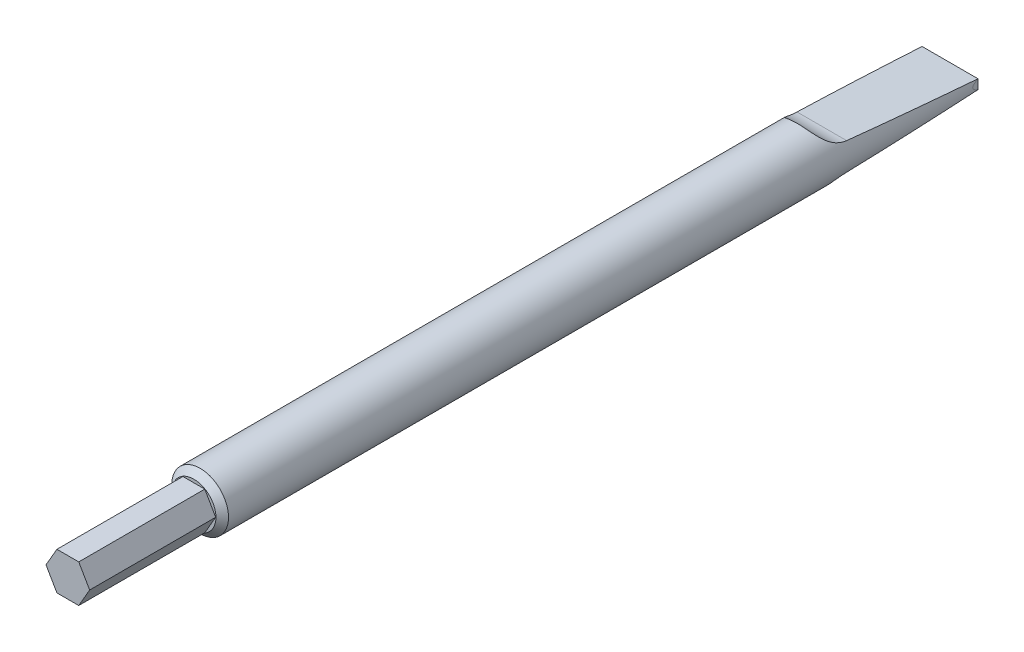
ISO-10303-21;
HEADER;
FILE_DESCRIPTION(('STEP AP214'),'2;1');
FILE_NAME('part.step','',(''),(''),'','','');
FILE_SCHEMA(('AUTOMOTIVE_DESIGN { 1 0 10303 214 1 1 1 1 }'));
ENDSEC;
DATA;
#1=APPLICATION_CONTEXT('core data for automotive mechanical design processes');
#2=APPLICATION_PROTOCOL_DEFINITION('international standard','automotive_design',2000,#1);
#3=PRODUCT_CONTEXT('',#1,'mechanical');
#4=PRODUCT('Part','Part','',(#3));
#5=PRODUCT_RELATED_PRODUCT_CATEGORY('part','',(#4));
#6=PRODUCT_DEFINITION_FORMATION('','',#4);
#7=PRODUCT_DEFINITION_CONTEXT('part definition',#1,'design');
#8=PRODUCT_DEFINITION('design','',#6,#7);
#9=PRODUCT_DEFINITION_SHAPE('','',#8);
#10=(LENGTH_UNIT() NAMED_UNIT(*) SI_UNIT(.MILLI.,.METRE.));
#11=(NAMED_UNIT(*) PLANE_ANGLE_UNIT() SI_UNIT($,.RADIAN.));
#12=(NAMED_UNIT(*) SI_UNIT($,.STERADIAN.) SOLID_ANGLE_UNIT());
#13=UNCERTAINTY_MEASURE_WITH_UNIT(LENGTH_MEASURE(1.E-05),#10,'distance_accuracy_value','');
#14=(GEOMETRIC_REPRESENTATION_CONTEXT(3) GLOBAL_UNCERTAINTY_ASSIGNED_CONTEXT((#13)) GLOBAL_UNIT_ASSIGNED_CONTEXT((#10,
#11,#12)) REPRESENTATION_CONTEXT('',''));
#15=CARTESIAN_POINT('',(0.,0.,0.));
#16=DIRECTION('',(0.,0.,1.));
#17=DIRECTION('',(1.,0.,0.));
#18=AXIS2_PLACEMENT_3D('',#15,#16,#17);
#19=CARTESIAN_POINT('',(0.,0.,-140.));
#20=DIRECTION('',(0.,0.,1.));
#21=DIRECTION('',(1.,0.,0.));
#22=AXIS2_PLACEMENT_3D('',#19,#20,#21);
#23=CYLINDRICAL_SURFACE('',#22,4.5);
#24=CARTESIAN_POINT('',(0.,0.,-21.));
#25=DIRECTION('',(0.,0.,1.));
#26=DIRECTION('',(1.,0.,0.));
#27=AXIS2_PLACEMENT_3D('',#24,#25,#26);
#28=CIRCLE('',#27,4.5);
#29=CARTESIAN_POINT('',(4.5,0.,-21.));
#30=VERTEX_POINT('',#29);
#31=EDGE_CURVE('E199',#30,#30,#28,.F.);
#32=ORIENTED_EDGE('',*,*,#31,.T.);
#33=EDGE_LOOP('',(#32));
#34=FACE_BOUND('',#33,.T.);
#35=CARTESIAN_POINT('',(0.,0.,-150.725499692534));
#36=DIRECTION('',(0.,-0.997564050259824,0.0697564737441254));
#37=DIRECTION('',(0.,0.0697564737441254,0.997564050259824));
#38=AXIS2_PLACEMENT_3D('',#35,#36,#37);
#39=ELLIPSE('',#38,64.5101416179165,4.5);
#40=CARTESIAN_POINT('',(4.43705983732471,0.75,-140.));
#41=VERTEX_POINT('',#40);
#42=CARTESIAN_POINT('',(3.94060843870063,2.17292547797695,-119.651217631279));
#43=VERTEX_POINT('',#42);
#44=EDGE_CURVE('E134',#41,#43,#39,.T.);
#45=ORIENTED_EDGE('',*,*,#44,.T.);
#46=CARTESIAN_POINT('',(3.94060843870063,2.17292547797695,-119.651217631279));
#47=CARTESIAN_POINT('',(3.93613453836127,2.18097697918258,-119.535820622681));
#48=CARTESIAN_POINT('',(3.92947094474121,2.19306262577348,-119.420781980209));
#49=CARTESIAN_POINT('',(3.91143990386196,2.22509503569858,-119.192142075211));
#50=CARTESIAN_POINT('',(3.90007100119166,2.24504423123616,-119.078541268641));
#51=CARTESIAN_POINT('',(3.87225058788964,2.29268834893347,-118.853110956475));
#52=CARTESIAN_POINT('',(3.8557785222487,2.32041455254767,-118.741290572735));
#53=CARTESIAN_POINT('',(3.81728624165493,2.38320927692897,-118.520713395312));
#54=CARTESIAN_POINT('',(3.7952665438402,2.41827711327371,-118.411956317124));
#55=CARTESIAN_POINT('',(3.74503067779343,2.49536896839162,-118.197992726652));
#56=CARTESIAN_POINT('',(3.71679509883591,2.53741467384938,-118.092798554982));
#57=CARTESIAN_POINT('',(3.65353870193094,2.62767774279538,-117.887206844789));
#58=CARTESIAN_POINT('',(3.61851845768965,2.6758945843401,-117.786808901595));
#59=CARTESIAN_POINT('',(3.54114938762096,2.77746734917336,-117.5919056934));
#60=CARTESIAN_POINT('',(3.49881744140523,2.8308113130091,-117.497387523424));
#61=CARTESIAN_POINT('',(3.40621740877894,2.94157932893592,-117.31485041299));
#62=CARTESIAN_POINT('',(3.35595018710472,2.99900293607863,-117.226830765896));
#63=CARTESIAN_POINT('',(3.2509131085579,3.11241176095055,-117.06399317642));
#64=CARTESIAN_POINT('',(3.19670952020653,3.16821355425757,-116.988682062981));
#65=CARTESIAN_POINT('',(3.08094814297472,3.28089601782652,-116.84482757073));
#66=CARTESIAN_POINT('',(3.01939113283397,3.33777657330996,-116.776283476681));
#67=CARTESIAN_POINT('',(2.88897355401037,3.45127540230262,-116.646304005054));
#68=CARTESIAN_POINT('',(2.82011348473832,3.50789369347048,-116.584868141988));
#69=CARTESIAN_POINT('',(2.67534804580783,3.61951134401522,-116.469261101259));
#70=CARTESIAN_POINT('',(2.59944311297892,3.67451080349253,-116.415089473671));
#71=CARTESIAN_POINT('',(2.44854074393229,3.77652535953582,-116.31876356579));
#72=CARTESIAN_POINT('',(2.37413558447831,3.82380378625174,-116.275957387855));
#73=CARTESIAN_POINT('',(2.22035176089097,3.9151035031153,-116.196122204785));
#74=CARTESIAN_POINT('',(2.1409714916143,3.95912373196058,-116.159095077761));
#75=CARTESIAN_POINT('',(1.97777084438874,4.04312355064204,-116.090604730084));
#76=CARTESIAN_POINT('',(1.89394932917378,4.08310209783241,-116.059142943579));
#77=CARTESIAN_POINT('',(1.72243379944664,4.15836458405134,-116.001505778205));
#78=CARTESIAN_POINT('',(1.63473840777443,4.19364683536831,-115.975332298059));
#79=CARTESIAN_POINT('',(1.45498290195123,4.25937769280764,-115.927687019373));
#80=CARTESIAN_POINT('',(1.36288173901448,4.28975985781964,-115.906278557151));
#81=CARTESIAN_POINT('',(1.1759495804635,4.34472539225634,-115.868275534781));
#82=CARTESIAN_POINT('',(1.08111733362925,4.36930605478777,-115.85168322095));
#83=CARTESIAN_POINT('',(0.889589599589855,4.41228344912634,-115.82308487023));
#84=CARTESIAN_POINT('',(0.792898196167833,4.43069239067199,-115.811069771572));
#85=CARTESIAN_POINT('',(0.598088772234088,4.46116654062827,-115.791365663627));
#86=CARTESIAN_POINT('',(0.499970875992387,4.47323229826743,-115.783676279791));
#87=CARTESIAN_POINT('',(0.334793464227263,4.48802810345971,-115.774289745482));
#88=CARTESIAN_POINT('',(0.267948323013006,4.49251523740662,-115.771459023129));
#89=CARTESIAN_POINT('',(0.13407114126273,4.49850140980018,-115.767687692857));
#90=CARTESIAN_POINT('',(0.0670390990430208,4.50000042124079,-115.766747102021));
#91=CARTESIAN_POINT('',(-0.103899728165749,4.4999993471451,-115.766746479842));
#92=CARTESIAN_POINT('',(-0.207816406800852,4.49639706128998,-115.769004812056));
#93=CARTESIAN_POINT('',(-0.414992715633222,4.48202756678654,-115.778088182435));
#94=CARTESIAN_POINT('',(-0.51825201929879,4.47125704115421,-115.784915334752));
#95=CARTESIAN_POINT('',(-0.723544595674429,4.44266135596965,-115.803298078138));
#96=CARTESIAN_POINT('',(-0.825575538970318,4.42482447219796,-115.814861528568));
#97=CARTESIAN_POINT('',(-1.02756052241239,4.38232527899109,-115.842954372874));
#98=CARTESIAN_POINT('',(-1.12751361949297,4.35765994004909,-115.859485971193));
#99=CARTESIAN_POINT('',(-1.32469006293437,4.30182602120851,-115.897838871514));
#100=CARTESIAN_POINT('',(-1.42190987280691,4.27064941973946,-115.919666703646));
#101=CARTESIAN_POINT('',(-1.61270615332902,4.2023137913944,-115.968939005443));
#102=CARTESIAN_POINT('',(-1.70628435417008,4.16515764968153,-115.996380768077));
#103=CARTESIAN_POINT('',(-1.88905676568278,4.0855103376416,-116.057229964812));
#104=CARTESIAN_POINT('',(-1.97825380865808,4.0430226788836,-116.090633478304));
#105=CARTESIAN_POINT('',(-2.15162802908161,3.9534813076382,-116.163752699636));
#106=CARTESIAN_POINT('',(-2.23580544578818,3.90642781306073,-116.203468106292));
#107=CARTESIAN_POINT('',(-2.39605028556675,3.81017251378525,-116.288175405829));
#108=CARTESIAN_POINT('',(-2.47228585911362,3.761078505754,-116.332971722124));
#109=CARTESIAN_POINT('',(-2.61898270302837,3.66044320005788,-116.428905771767));
#110=CARTESIAN_POINT('',(-2.68944197304487,3.60890106427654,-116.480045686644));
#111=CARTESIAN_POINT('',(-2.82415599278798,3.50448332513091,-116.588634634983));
#112=CARTESIAN_POINT('',(-2.88841415937434,3.45160847659475,-116.646080156272));
#113=CARTESIAN_POINT('',(-3.01058224303268,3.3455851685044,-116.767195132878));
#114=CARTESIAN_POINT('',(-3.0684898196607,3.29243661558388,-116.830866866557));
#115=CARTESIAN_POINT('',(-3.17574329962985,3.18904171265143,-116.961540598027));
#116=CARTESIAN_POINT('',(-3.22533513488353,3.13876304771544,-117.02831565721));
#117=CARTESIAN_POINT('',(-3.31869480646399,3.03988341659307,-117.167024542179));
#118=CARTESIAN_POINT('',(-3.3624605753757,2.99128305046796,-117.238960185368));
#119=CARTESIAN_POINT('',(-3.44435200258205,2.89661152472469,-117.387545271136));
#120=CARTESIAN_POINT('',(-3.48247761883405,2.85054038396139,-117.464194748846));
#121=CARTESIAN_POINT('',(-3.5533922834407,2.76163697617393,-117.621759266709));
#122=CARTESIAN_POINT('',(-3.58617934656772,2.71880591718232,-117.702675878924));
#123=CARTESIAN_POINT('',(-3.64844684895386,2.63471555664881,-117.872898609567));
#124=CARTESIAN_POINT('',(-3.67763825368493,2.59367954418583,-117.962420683473));
#125=CARTESIAN_POINT('',(-3.73087847262744,2.51649461313893,-118.145069383353));
#126=CARTESIAN_POINT('',(-3.75492510540121,2.48034776999426,-118.238197518649));
#127=CARTESIAN_POINT('',(-3.79828256501097,2.41342928729884,-118.427405808864));
#128=CARTESIAN_POINT('',(-3.8175946756726,2.38265619124115,-118.523485155555));
#129=CARTESIAN_POINT('',(-3.85188091079617,2.32681768893628,-118.718051853066));
#130=CARTESIAN_POINT('',(-3.86685449345663,2.30175299564602,-118.816539502974));
#131=CARTESIAN_POINT('',(-3.89557075715267,2.25289241108845,-119.036560045232));
#132=CARTESIAN_POINT('',(-3.90837111115832,2.23050520402001,-119.158531278134));
#133=CARTESIAN_POINT('',(-3.92848003713233,2.19484953417759,-119.403943849301));
#134=CARTESIAN_POINT('',(-3.935801859481,2.18155907668645,-119.527380902224));
#135=CARTESIAN_POINT('',(-3.94060843870063,2.17292547797695,-119.651217631279));
#136=B_SPLINE_CURVE_WITH_KNOTS('',3,(#46,#47,#48,#49,#50,#51,#52,#53,#54,#55,#56,#57,#58,#59,
#60,#61,#62,#63,#64,#65,#66,#67,#68,#69,#70,#71,#72,#73,#74,#75,#76,#77,#78,#79,#80,#81,#82,#83,
#84,#85,#86,#87,#88,#89,#90,#91,#92,#93,#94,#95,#96,#97,#98,#99,#100,#101,#102,#103,#104,#105,
#106,#107,#108,#109,#110,#111,#112,#113,#114,#115,#116,#117,#118,#119,#120,#121,#122,#123,#124,
#125,#126,#127,#128,#129,#130,#131,#132,#133,#134,#135),.UNSPECIFIED.,.F.,.F.,(4,2,2,2,2,2,2,2,
2,2,2,2,2,2,2,2,2,2,2,2,2,2,2,2,2,2,2,2,2,2,2,2,2,2,2,2,2,2,2,2,2,2,2,2,4),(0.,
0.347213481850569,0.694534441545247,1.04327297331349,1.39197900846225,1.74178981927731,
2.0915710632544,2.44055534800832,2.78950162887225,3.11387755351365,3.43821915660431,
3.76253859427388,4.0868379353466,4.38048652057452,4.67423033967267,4.96804974448696,
5.26197445596484,5.55959931971795,5.85736277740991,6.15453363404642,6.45167875571977,
6.65275701811363,6.85383709780358,7.16547860130777,7.47726441210352,7.78956970663768,
8.10201378094384,8.41484506654002,8.72752585929503,9.0400017773417,9.35246278943322,
9.65548728912214,9.95861628768749,10.2615772943742,10.5646495816183,10.8558942484657,
11.1472419913092,11.4385919057976,11.7300499172571,12.0378731212137,12.3458265879224,
12.6536964565557,12.9616047558562,13.3351302308025,13.7077493504199),.UNSPECIFIED.);
#137=CARTESIAN_POINT('',(-3.94060843870063,2.17292547797695,-119.651217631279));
#138=VERTEX_POINT('',#137);
#139=EDGE_CURVE('E12',#43,#138,#136,.T.);
#140=ORIENTED_EDGE('',*,*,#139,.T.);
#141=CARTESIAN_POINT('',(-4.43705983732471,0.75,-140.));
#142=VERTEX_POINT('',#141);
#143=EDGE_CURVE('E127',#138,#142,#39,.T.);
#144=ORIENTED_EDGE('',*,*,#143,.T.);
#145=CARTESIAN_POINT('',(0.,0.,-203.452911894641));
#146=DIRECTION('',(0.997564050259824,0.,0.0697564737441254));
#147=DIRECTION('',(-0.0697564737441254,0.,0.997564050259824));
#148=AXIS2_PLACEMENT_3D('',#145,#146,#147);
#149=ELLIPSE('',#148,64.5101416179165,4.5);
#150=CARTESIAN_POINT('',(-4.43705983732471,-0.75,-140.));
#151=VERTEX_POINT('',#150);
#152=EDGE_CURVE('E129',#142,#151,#149,.T.);
#153=ORIENTED_EDGE('',*,*,#152,.T.);
#154=CARTESIAN_POINT('',(0.,0.,-150.725499692534));
#155=DIRECTION('',(0.,0.997564050259824,0.0697564737441254));
#156=DIRECTION('',(0.,-0.0697564737441254,0.997564050259824));
#157=AXIS2_PLACEMENT_3D('',#154,#155,#156);
#158=ELLIPSE('',#157,64.5101416179165,4.5);
#159=CARTESIAN_POINT('',(-3.94060843870063,-2.17292547797695,-119.651217631279));
#160=VERTEX_POINT('',#159);
#161=EDGE_CURVE('E78',#151,#160,#158,.T.);
#162=ORIENTED_EDGE('',*,*,#161,.T.);
#163=CARTESIAN_POINT('',(-3.94060843870063,-2.17292547797695,-119.651217631279));
#164=CARTESIAN_POINT('',(-3.93613453836127,-2.18097697918258,-119.535820622681));
#165=CARTESIAN_POINT('',(-3.92947094474121,-2.19306262577348,-119.420781980209));
#166=CARTESIAN_POINT('',(-3.91143990386196,-2.22509503569858,-119.192142075211));
#167=CARTESIAN_POINT('',(-3.90007100119166,-2.24504423123616,-119.078541268641));
#168=CARTESIAN_POINT('',(-3.87225058788964,-2.29268834893347,-118.853110956475));
#169=CARTESIAN_POINT('',(-3.8557785222487,-2.32041455254767,-118.741290572735));
#170=CARTESIAN_POINT('',(-3.81728624165493,-2.38320927692897,-118.520713395312));
#171=CARTESIAN_POINT('',(-3.7952665438402,-2.41827711327371,-118.411956317124));
#172=CARTESIAN_POINT('',(-3.74503067779343,-2.49536896839162,-118.197992726652));
#173=CARTESIAN_POINT('',(-3.71679509883591,-2.53741467384938,-118.092798554982));
#174=CARTESIAN_POINT('',(-3.65353870193094,-2.62767774279538,-117.887206844789));
#175=CARTESIAN_POINT('',(-3.61851845768965,-2.6758945843401,-117.786808901595));
#176=CARTESIAN_POINT('',(-3.54114938762096,-2.77746734917336,-117.5919056934));
#177=CARTESIAN_POINT('',(-3.49881744140523,-2.8308113130091,-117.497387523424));
#178=CARTESIAN_POINT('',(-3.40621740877894,-2.94157932893592,-117.31485041299));
#179=CARTESIAN_POINT('',(-3.35595018710472,-2.99900293607863,-117.226830765896));
#180=CARTESIAN_POINT('',(-3.2509131085579,-3.11241176095055,-117.06399317642));
#181=CARTESIAN_POINT('',(-3.19670952020653,-3.16821355425757,-116.988682062981));
#182=CARTESIAN_POINT('',(-3.08094814297472,-3.28089601782652,-116.84482757073));
#183=CARTESIAN_POINT('',(-3.01939113283397,-3.33777657330996,-116.776283476681));
#184=CARTESIAN_POINT('',(-2.88897355401037,-3.45127540230262,-116.646304005054));
#185=CARTESIAN_POINT('',(-2.82011348473832,-3.50789369347048,-116.584868141988));
#186=CARTESIAN_POINT('',(-2.67534804580783,-3.61951134401522,-116.469261101259));
#187=CARTESIAN_POINT('',(-2.59944311297892,-3.67451080349253,-116.415089473671));
#188=CARTESIAN_POINT('',(-2.44854074393229,-3.77652535953582,-116.31876356579));
#189=CARTESIAN_POINT('',(-2.37413558447831,-3.82380378625174,-116.275957387855));
#190=CARTESIAN_POINT('',(-2.22035176089097,-3.9151035031153,-116.196122204785));
#191=CARTESIAN_POINT('',(-2.1409714916143,-3.95912373196058,-116.159095077761));
#192=CARTESIAN_POINT('',(-1.97777084438874,-4.04312355064204,-116.090604730084));
#193=CARTESIAN_POINT('',(-1.89394932917378,-4.08310209783241,-116.059142943579));
#194=CARTESIAN_POINT('',(-1.72243379944664,-4.15836458405134,-116.001505778205));
#195=CARTESIAN_POINT('',(-1.63473840777443,-4.19364683536831,-115.975332298059));
#196=CARTESIAN_POINT('',(-1.45498290195123,-4.25937769280764,-115.927687019373));
#197=CARTESIAN_POINT('',(-1.36288173901448,-4.28975985781964,-115.906278557151));
#198=CARTESIAN_POINT('',(-1.1759495804635,-4.34472539225634,-115.868275534781));
#199=CARTESIAN_POINT('',(-1.08111733362925,-4.36930605478777,-115.85168322095));
#200=CARTESIAN_POINT('',(-0.889589599589855,-4.41228344912634,-115.82308487023));
#201=CARTESIAN_POINT('',(-0.792898196167832,-4.43069239067199,-115.811069771572));
#202=CARTESIAN_POINT('',(-0.598088772234087,-4.46116654062827,-115.791365663627));
#203=CARTESIAN_POINT('',(-0.499970875992387,-4.47323229826743,-115.783676279791));
#204=CARTESIAN_POINT('',(-0.334793464227263,-4.48802810345971,-115.774289745482));
#205=CARTESIAN_POINT('',(-0.267948323013006,-4.49251523740662,-115.771459023129));
#206=CARTESIAN_POINT('',(-0.13407114126273,-4.49850140980018,-115.767687692857));
#207=CARTESIAN_POINT('',(-0.0670390990430203,-4.50000042124079,-115.766747102021));
#208=CARTESIAN_POINT('',(0.103899728165749,-4.4999993471451,-115.766746479842));
#209=CARTESIAN_POINT('',(0.207816406800852,-4.49639706128998,-115.769004812056));
#210=CARTESIAN_POINT('',(0.414992715633222,-4.48202756678654,-115.778088182435));
#211=CARTESIAN_POINT('',(0.518252019298791,-4.47125704115421,-115.784915334752));
#212=CARTESIAN_POINT('',(0.72354459567443,-4.44266135596965,-115.803298078138));
#213=CARTESIAN_POINT('',(0.825575538970319,-4.42482447219796,-115.814861528568));
#214=CARTESIAN_POINT('',(1.02756052241239,-4.38232527899109,-115.842954372874));
#215=CARTESIAN_POINT('',(1.12751361949297,-4.35765994004909,-115.859485971193));
#216=CARTESIAN_POINT('',(1.32469006293437,-4.30182602120851,-115.897838871514));
#217=CARTESIAN_POINT('',(1.42190987280691,-4.27064941973946,-115.919666703646));
#218=CARTESIAN_POINT('',(1.61270615332902,-4.2023137913944,-115.968939005443));
#219=CARTESIAN_POINT('',(1.70628435417008,-4.16515764968153,-115.996380768077));
#220=CARTESIAN_POINT('',(1.88905676568278,-4.0855103376416,-116.057229964812));
#221=CARTESIAN_POINT('',(1.97825380865808,-4.0430226788836,-116.090633478304));
#222=CARTESIAN_POINT('',(2.15162802908161,-3.9534813076382,-116.163752699636));
#223=CARTESIAN_POINT('',(2.23580544578818,-3.90642781306073,-116.203468106292));
#224=CARTESIAN_POINT('',(2.39605028556675,-3.81017251378525,-116.288175405829));
#225=CARTESIAN_POINT('',(2.47228585911362,-3.761078505754,-116.332971722124));
#226=CARTESIAN_POINT('',(2.61898270302837,-3.66044320005788,-116.428905771767));
#227=CARTESIAN_POINT('',(2.68944197304487,-3.60890106427654,-116.480045686644));
#228=CARTESIAN_POINT('',(2.82415599278798,-3.50448332513091,-116.588634634983));
#229=CARTESIAN_POINT('',(2.88841415937434,-3.45160847659476,-116.646080156272));
#230=CARTESIAN_POINT('',(3.01058224303268,-3.34558516850441,-116.767195132878));
#231=CARTESIAN_POINT('',(3.0684898196607,-3.29243661558389,-116.830866866557));
#232=CARTESIAN_POINT('',(3.17574329962985,-3.18904171265143,-116.961540598027));
#233=CARTESIAN_POINT('',(3.22533513488353,-3.13876304771544,-117.02831565721));
#234=CARTESIAN_POINT('',(3.31869480646398,-3.03988341659307,-117.167024542179));
#235=CARTESIAN_POINT('',(3.3624605753757,-2.99128305046797,-117.238960185368));
#236=CARTESIAN_POINT('',(3.44435200258205,-2.89661152472469,-117.387545271136));
#237=CARTESIAN_POINT('',(3.48247761883405,-2.85054038396139,-117.464194748846));
#238=CARTESIAN_POINT('',(3.5533922834407,-2.76163697617393,-117.621759266709));
#239=CARTESIAN_POINT('',(3.58617934656772,-2.71880591718232,-117.702675878924));
#240=CARTESIAN_POINT('',(3.64844684895386,-2.63471555664882,-117.872898609567));
#241=CARTESIAN_POINT('',(3.67763825368493,-2.59367954418584,-117.962420683473));
#242=CARTESIAN_POINT('',(3.73087847262744,-2.51649461313893,-118.145069383353));
#243=CARTESIAN_POINT('',(3.75492510540121,-2.48034776999426,-118.238197518649));
#244=CARTESIAN_POINT('',(3.79828256501097,-2.41342928729884,-118.427405808864));
#245=CARTESIAN_POINT('',(3.8175946756726,-2.38265619124115,-118.523485155555));
#246=CARTESIAN_POINT('',(3.85188091079616,-2.32681768893628,-118.718051853066));
#247=CARTESIAN_POINT('',(3.86685449345663,-2.30175299564602,-118.816539502974));
#248=CARTESIAN_POINT('',(3.89557075715267,-2.25289241108845,-119.036560045232));
#249=CARTESIAN_POINT('',(3.90837111115832,-2.23050520402001,-119.158531278134));
#250=CARTESIAN_POINT('',(3.92848003713233,-2.19484953417759,-119.403943849301));
#251=CARTESIAN_POINT('',(3.935801859481,-2.18155907668645,-119.527380902224));
#252=CARTESIAN_POINT('',(3.94060843870063,-2.17292547797695,-119.651217631279));
#253=B_SPLINE_CURVE_WITH_KNOTS('',3,(#163,#164,#165,#166,#167,#168,#169,#170,#171,#172,#173,
#174,#175,#176,#177,#178,#179,#180,#181,#182,#183,#184,#185,#186,#187,#188,#189,#190,#191,#192,
#193,#194,#195,#196,#197,#198,#199,#200,#201,#202,#203,#204,#205,#206,#207,#208,#209,#210,#211,
#212,#213,#214,#215,#216,#217,#218,#219,#220,#221,#222,#223,#224,#225,#226,#227,#228,#229,#230,
#231,#232,#233,#234,#235,#236,#237,#238,#239,#240,#241,#242,#243,#244,#245,#246,#247,#248,#249,
#250,#251,#252),.UNSPECIFIED.,.F.,.F.,(4,2,2,2,2,2,2,2,2,2,2,2,2,2,2,2,2,2,2,2,2,2,2,2,2,2,2,2,
2,2,2,2,2,2,2,2,2,2,2,2,2,2,2,2,4),(0.,0.347213481850569,0.694534441545247,1.04327297331349,
1.39197900846225,1.74178981927731,2.0915710632544,2.44055534800832,2.78950162887225,
3.11387755351365,3.43821915660431,3.76253859427388,4.0868379353466,4.38048652057452,
4.67423033967267,4.96804974448696,5.26197445596484,5.55959931971795,5.85736277740991,
6.15453363404642,6.45167875571977,6.65275701811363,6.85383709780358,7.16547860130777,
7.47726441210352,7.78956970663768,8.10201378094384,8.41484506654002,8.72752585929503,
9.0400017773417,9.35246278943322,9.65548728912214,9.95861628768749,10.2615772943742,
10.5646495816183,10.8558942484657,11.1472419913092,11.4385919057976,11.7300499172571,
12.0378731212137,12.3458265879224,12.6536964565556,12.9616047558562,13.3351302308026,
13.7077493504199),.UNSPECIFIED.);
#254=CARTESIAN_POINT('',(3.94060843870063,-2.17292547797695,-119.651217631279));
#255=VERTEX_POINT('',#254);
#256=EDGE_CURVE('E59',#160,#255,#253,.T.);
#257=ORIENTED_EDGE('',*,*,#256,.T.);
#258=CARTESIAN_POINT('',(4.43705983732471,-0.75,-140.));
#259=VERTEX_POINT('',#258);
#260=EDGE_CURVE('E145',#255,#259,#158,.T.);
#261=ORIENTED_EDGE('',*,*,#260,.T.);
#262=CARTESIAN_POINT('',(0.,0.,-203.452911894641));
#263=DIRECTION('',(-0.997564050259824,0.,0.0697564737441254));
#264=DIRECTION('',(0.0697564737441254,0.,0.997564050259824));
#265=AXIS2_PLACEMENT_3D('',#262,#263,#264);
#266=ELLIPSE('',#265,64.5101416179165,4.5);
#267=EDGE_CURVE('E131',#259,#41,#266,.T.);
#268=ORIENTED_EDGE('',*,*,#267,.T.);
#269=EDGE_LOOP('',(#45,#140,#144,#153,#162,#257,#261,#268));
#270=FACE_BOUND('',#269,.T.);
#271=ADVANCED_FACE('F43',(#34,#270),#23,.T.);
#272=CARTESIAN_POINT('',(0.,0.,-20.));
#273=DIRECTION('',(0.,0.,1.));
#274=DIRECTION('',(1.,0.,0.));
#275=AXIS2_PLACEMENT_3D('',#272,#273,#274);
#276=PLANE('',#275);
#277=CARTESIAN_POINT('',(0.,0.,-20.));
#278=DIRECTION('',(0.,0.,1.));
#279=DIRECTION('',(1.,0.,0.));
#280=AXIS2_PLACEMENT_3D('',#277,#278,#279);
#281=CIRCLE('',#280,3.50000000000001);
#282=CARTESIAN_POINT('',(3.50000000000001,0.,-20.));
#283=VERTEX_POINT('',#282);
#284=EDGE_CURVE('E215',#283,#283,#281,.T.);
#285=ORIENTED_EDGE('',*,*,#284,.T.);
#286=EDGE_LOOP('',(#285));
#287=FACE_BOUND('',#286,.T.);
#288=DIRECTION('',(1.,0.,0.));
#289=VECTOR('',#288,1.);
#290=CARTESIAN_POINT('',(-1.73205080756888,-3.,-20.));
#291=LINE('',#290,#289);
#292=CARTESIAN_POINT('',(-1.73205080756888,-3.,-20.));
#293=VERTEX_POINT('',#292);
#294=CARTESIAN_POINT('',(1.73205080756888,-3.,-20.));
#295=VERTEX_POINT('',#294);
#296=EDGE_CURVE('E180',#293,#295,#291,.T.);
#297=ORIENTED_EDGE('',*,*,#296,.F.);
#298=DIRECTION('',(0.5,-0.866025403784439,0.));
#299=VECTOR('',#298,1.);
#300=CARTESIAN_POINT('',(-3.46410161513775,0.,-20.));
#301=LINE('',#300,#299);
#302=CARTESIAN_POINT('',(-3.46410161513775,0.,-20.));
#303=VERTEX_POINT('',#302);
#304=EDGE_CURVE('E172',#303,#293,#301,.T.);
#305=ORIENTED_EDGE('',*,*,#304,.F.);
#306=DIRECTION('',(-0.5,-0.866025403784439,0.));
#307=VECTOR('',#306,1.);
#308=CARTESIAN_POINT('',(-1.73205080756888,3.,-20.));
#309=LINE('',#308,#307);
#310=CARTESIAN_POINT('',(-1.73205080756888,3.,-20.));
#311=VERTEX_POINT('',#310);
#312=EDGE_CURVE('E171',#311,#303,#309,.T.);
#313=ORIENTED_EDGE('',*,*,#312,.F.);
#314=DIRECTION('',(-1.,0.,0.));
#315=VECTOR('',#314,1.);
#316=CARTESIAN_POINT('',(1.73205080756888,3.,-20.));
#317=LINE('',#316,#315);
#318=CARTESIAN_POINT('',(1.73205080756888,3.,-20.));
#319=VERTEX_POINT('',#318);
#320=EDGE_CURVE('E166',#319,#311,#317,.T.);
#321=ORIENTED_EDGE('',*,*,#320,.F.);
#322=DIRECTION('',(-0.5,0.866025403784438,0.));
#323=VECTOR('',#322,1.);
#324=CARTESIAN_POINT('',(3.46410161513776,0.,-20.));
#325=LINE('',#324,#323);
#326=CARTESIAN_POINT('',(3.46410161513776,0.,-20.));
#327=VERTEX_POINT('',#326);
#328=EDGE_CURVE('E165',#327,#319,#325,.T.);
#329=ORIENTED_EDGE('',*,*,#328,.F.);
#330=DIRECTION('',(0.5,0.866025403784439,0.));
#331=VECTOR('',#330,1.);
#332=CARTESIAN_POINT('',(1.73205080756888,-3.,-20.));
#333=LINE('',#332,#331);
#334=EDGE_CURVE('E163',#295,#327,#333,.T.);
#335=ORIENTED_EDGE('',*,*,#334,.F.);
#336=EDGE_LOOP('',(#297,#305,#313,#321,#329,#335));
#337=FACE_BOUND('',#336,.T.);
#338=ADVANCED_FACE('F226',(#287,#337),#276,.T.);
#339=CARTESIAN_POINT('',(1.73205080756888,-3.,-20.));
#340=DIRECTION('',(0.866025403784439,-0.5,0.));
#341=DIRECTION('',(0.5,0.866025403784439,0.));
#342=AXIS2_PLACEMENT_3D('',#339,#340,#341);
#343=PLANE('',#342);
#344=DIRECTION('',(0.5,0.866025403784439,0.));
#345=VECTOR('',#344,1.);
#346=CARTESIAN_POINT('',(1.73205080756888,-3.,0.));
#347=LINE('',#346,#345);
#348=CARTESIAN_POINT('',(1.73205080756888,-3.,0.));
#349=VERTEX_POINT('',#348);
#350=CARTESIAN_POINT('',(3.46410161513775,0.,0.));
#351=VERTEX_POINT('',#350);
#352=EDGE_CURVE('E142',#349,#351,#347,.T.);
#353=ORIENTED_EDGE('',*,*,#352,.F.);
#354=DIRECTION('',(0.,0.,1.));
#355=VECTOR('',#354,1.);
#356=CARTESIAN_POINT('',(1.73205080756888,-3.,-20.));
#357=LINE('',#356,#355);
#358=EDGE_CURVE('E200',#295,#349,#357,.T.);
#359=ORIENTED_EDGE('',*,*,#358,.F.);
#360=ORIENTED_EDGE('',*,*,#334,.T.);
#361=DIRECTION('',(0.,0.,1.));
#362=VECTOR('',#361,1.);
#363=CARTESIAN_POINT('',(3.46410161513776,0.,-20.));
#364=LINE('',#363,#362);
#365=EDGE_CURVE('E179',#327,#351,#364,.T.);
#366=ORIENTED_EDGE('',*,*,#365,.T.);
#367=EDGE_LOOP('',(#353,#359,#360,#366));
#368=FACE_BOUND('',#367,.T.);
#369=ADVANCED_FACE('F251',(#368),#343,.T.);
#370=CARTESIAN_POINT('',(-1.73205080756888,-3.,-20.));
#371=DIRECTION('',(0.,-1.,0.));
#372=DIRECTION('',(0.,0.,-1.));
#373=AXIS2_PLACEMENT_3D('',#370,#371,#372);
#374=PLANE('',#373);
#375=DIRECTION('',(1.,0.,0.));
#376=VECTOR('',#375,1.);
#377=CARTESIAN_POINT('',(-1.73205080756888,-3.,0.));
#378=LINE('',#377,#376);
#379=CARTESIAN_POINT('',(-1.73205080756888,-3.,0.));
#380=VERTEX_POINT('',#379);
#381=EDGE_CURVE('E164',#380,#349,#378,.T.);
#382=ORIENTED_EDGE('',*,*,#381,.F.);
#383=DIRECTION('',(0.,0.,1.));
#384=VECTOR('',#383,1.);
#385=CARTESIAN_POINT('',(-1.73205080756888,-3.,-20.));
#386=LINE('',#385,#384);
#387=EDGE_CURVE('E197',#293,#380,#386,.T.);
#388=ORIENTED_EDGE('',*,*,#387,.F.);
#389=ORIENTED_EDGE('',*,*,#296,.T.);
#390=ORIENTED_EDGE('',*,*,#358,.T.);
#391=EDGE_LOOP('',(#382,#388,#389,#390));
#392=FACE_BOUND('',#391,.T.);
#393=ADVANCED_FACE('F277',(#392),#374,.T.);
#394=CARTESIAN_POINT('',(-3.46410161513775,0.,-20.));
#395=DIRECTION('',(-0.866025403784438,-0.5,0.));
#396=DIRECTION('',(0.5,-0.866025403784439,0.));
#397=AXIS2_PLACEMENT_3D('',#394,#395,#396);
#398=PLANE('',#397);
#399=DIRECTION('',(0.5,-0.866025403784439,0.));
#400=VECTOR('',#399,1.);
#401=CARTESIAN_POINT('',(-3.46410161513775,0.,0.));
#402=LINE('',#401,#400);
#403=CARTESIAN_POINT('',(-3.46410161513775,0.,0.));
#404=VERTEX_POINT('',#403);
#405=EDGE_CURVE('E195',#404,#380,#402,.T.);
#406=ORIENTED_EDGE('',*,*,#405,.F.);
#407=DIRECTION('',(0.,0.,1.));
#408=VECTOR('',#407,1.);
#409=CARTESIAN_POINT('',(-3.46410161513775,0.,-20.));
#410=LINE('',#409,#408);
#411=EDGE_CURVE('E205',#303,#404,#410,.T.);
#412=ORIENTED_EDGE('',*,*,#411,.F.);
#413=ORIENTED_EDGE('',*,*,#304,.T.);
#414=ORIENTED_EDGE('',*,*,#387,.T.);
#415=EDGE_LOOP('',(#406,#412,#413,#414));
#416=FACE_BOUND('',#415,.T.);
#417=ADVANCED_FACE('F264',(#416),#398,.T.);
#418=CARTESIAN_POINT('',(-1.73205080756888,3.,-20.));
#419=DIRECTION('',(-0.866025403784439,0.5,0.));
#420=DIRECTION('',(-0.5,-0.866025403784439,0.));
#421=AXIS2_PLACEMENT_3D('',#418,#419,#420);
#422=PLANE('',#421);
#423=DIRECTION('',(-0.5,-0.866025403784439,0.));
#424=VECTOR('',#423,1.);
#425=CARTESIAN_POINT('',(-1.73205080756888,3.,0.));
#426=LINE('',#425,#424);
#427=CARTESIAN_POINT('',(-1.73205080756888,3.,0.));
#428=VERTEX_POINT('',#427);
#429=EDGE_CURVE('E186',#428,#404,#426,.T.);
#430=ORIENTED_EDGE('',*,*,#429,.F.);
#431=DIRECTION('',(0.,0.,1.));
#432=VECTOR('',#431,1.);
#433=CARTESIAN_POINT('',(-1.73205080756888,3.,-20.));
#434=LINE('',#433,#432);
#435=EDGE_CURVE('E204',#311,#428,#434,.T.);
#436=ORIENTED_EDGE('',*,*,#435,.F.);
#437=ORIENTED_EDGE('',*,*,#312,.T.);
#438=ORIENTED_EDGE('',*,*,#411,.T.);
#439=EDGE_LOOP('',(#430,#436,#437,#438));
#440=FACE_BOUND('',#439,.T.);
#441=ADVANCED_FACE('F266',(#440),#422,.T.);
#442=CARTESIAN_POINT('',(1.73205080756888,3.,-20.));
#443=DIRECTION('',(0.,1.,0.));
#444=DIRECTION('',(0.,0.,1.));
#445=AXIS2_PLACEMENT_3D('',#442,#443,#444);
#446=PLANE('',#445);
#447=DIRECTION('',(-1.,0.,0.));
#448=VECTOR('',#447,1.);
#449=CARTESIAN_POINT('',(1.73205080756888,3.,0.));
#450=LINE('',#449,#448);
#451=CARTESIAN_POINT('',(1.73205080756888,3.,0.));
#452=VERTEX_POINT('',#451);
#453=EDGE_CURVE('E187',#452,#428,#450,.T.);
#454=ORIENTED_EDGE('',*,*,#453,.F.);
#455=DIRECTION('',(0.,0.,1.));
#456=VECTOR('',#455,1.);
#457=CARTESIAN_POINT('',(1.73205080756888,3.,-20.));
#458=LINE('',#457,#456);
#459=EDGE_CURVE('E207',#319,#452,#458,.T.);
#460=ORIENTED_EDGE('',*,*,#459,.F.);
#461=ORIENTED_EDGE('',*,*,#320,.T.);
#462=ORIENTED_EDGE('',*,*,#435,.T.);
#463=EDGE_LOOP('',(#454,#460,#461,#462));
#464=FACE_BOUND('',#463,.T.);
#465=ADVANCED_FACE('F272',(#464),#446,.T.);
#466=CARTESIAN_POINT('',(3.46410161513776,0.,-20.));
#467=DIRECTION('',(0.866025403784438,0.5,0.));
#468=DIRECTION('',(-0.5,0.866025403784439,0.));
#469=AXIS2_PLACEMENT_3D('',#466,#467,#468);
#470=PLANE('',#469);
#471=DIRECTION('',(-0.5,0.866025403784438,0.));
#472=VECTOR('',#471,1.);
#473=CARTESIAN_POINT('',(3.46410161513776,0.,0.));
#474=LINE('',#473,#472);
#475=EDGE_CURVE('E182',#351,#452,#474,.T.);
#476=ORIENTED_EDGE('',*,*,#475,.F.);
#477=ORIENTED_EDGE('',*,*,#365,.F.);
#478=ORIENTED_EDGE('',*,*,#328,.T.);
#479=ORIENTED_EDGE('',*,*,#459,.T.);
#480=EDGE_LOOP('',(#476,#477,#478,#479));
#481=FACE_BOUND('',#480,.T.);
#482=ADVANCED_FACE('F250',(#481),#470,.T.);
#483=CARTESIAN_POINT('',(0.,0.,0.));
#484=DIRECTION('',(0.,0.,1.));
#485=DIRECTION('',(1.,0.,0.));
#486=AXIS2_PLACEMENT_3D('',#483,#484,#485);
#487=PLANE('',#486);
#488=ORIENTED_EDGE('',*,*,#381,.T.);
#489=ORIENTED_EDGE('',*,*,#352,.T.);
#490=ORIENTED_EDGE('',*,*,#475,.T.);
#491=ORIENTED_EDGE('',*,*,#453,.T.);
#492=ORIENTED_EDGE('',*,*,#429,.T.);
#493=ORIENTED_EDGE('',*,*,#405,.T.);
#494=EDGE_LOOP('',(#488,#489,#490,#491,#492,#493));
#495=FACE_BOUND('',#494,.T.);
#496=ADVANCED_FACE('F229',(#495),#487,.T.);
#497=CARTESIAN_POINT('',(0.,0.,-21.));
#498=DIRECTION('',(0.,0.,-1.));
#499=DIRECTION('',(-1.,0.,0.));
#500=AXIS2_PLACEMENT_3D('',#497,#498,#499);
#501=CONICAL_SURFACE('',#500,4.5,0.785398163397453);
#502=ORIENTED_EDGE('',*,*,#284,.F.);
#503=EDGE_LOOP('',(#502));
#504=FACE_BOUND('',#503,.T.);
#505=ORIENTED_EDGE('',*,*,#31,.F.);
#506=EDGE_LOOP('',(#505));
#507=FACE_BOUND('',#506,.T.);
#508=ADVANCED_FACE('F231',(#504,#507),#501,.T.);
#509=CARTESIAN_POINT('',(4.43705983732471,0.75,-140.));
#510=DIRECTION('',(0.,-0.997564050259824,0.0697564737441254));
#511=DIRECTION('',(0.,-0.0697564737441254,-0.997564050259824));
#512=AXIS2_PLACEMENT_3D('',#509,#510,#511);
#513=PLANE('',#512);
#514=ORIENTED_EDGE('',*,*,#143,.F.);
#515=DIRECTION('',(1.,0.,0.));
#516=VECTOR('',#515,1.);
#517=CARTESIAN_POINT('',(3.74287926057653,2.17292547797695,-119.651217631279));
#518=LINE('',#517,#516);
#519=EDGE_CURVE('E220',#138,#43,#518,.T.);
#520=ORIENTED_EDGE('',*,*,#519,.T.);
#521=ORIENTED_EDGE('',*,*,#44,.F.);
#522=DIRECTION('',(1.,0.,0.));
#523=VECTOR('',#522,1.);
#524=CARTESIAN_POINT('',(4.43705983732471,0.75,-140.));
#525=LINE('',#524,#523);
#526=EDGE_CURVE('E147',#142,#41,#525,.T.);
#527=ORIENTED_EDGE('',*,*,#526,.F.);
#528=EDGE_LOOP('',(#514,#520,#521,#527));
#529=FACE_BOUND('',#528,.T.);
#530=ADVANCED_FACE('F150',(#529),#513,.F.);
#531=CARTESIAN_POINT('',(4.43705983732471,-0.75,-140.));
#532=DIRECTION('',(-0.997564050259824,0.,0.0697564737441254));
#533=DIRECTION('',(0.0697564737441254,0.,0.997564050259824));
#534=AXIS2_PLACEMENT_3D('',#531,#532,#533);
#535=PLANE('',#534);
#536=DIRECTION('',(0.,-1.,0.));
#537=VECTOR('',#536,1.);
#538=CARTESIAN_POINT('',(4.43705983732471,-0.75,-140.));
#539=LINE('',#538,#537);
#540=EDGE_CURVE('E153',#41,#259,#539,.T.);
#541=ORIENTED_EDGE('',*,*,#540,.F.);
#542=ORIENTED_EDGE('',*,*,#267,.F.);
#543=EDGE_LOOP('',(#541,#542));
#544=FACE_BOUND('',#543,.T.);
#545=ADVANCED_FACE('F242',(#544),#535,.F.);
#546=CARTESIAN_POINT('',(4.43705983732471,-0.75,-140.));
#547=DIRECTION('',(0.,0.997564050259824,0.0697564737441254));
#548=DIRECTION('',(0.,-0.0697564737441254,0.997564050259824));
#549=AXIS2_PLACEMENT_3D('',#546,#547,#548);
#550=PLANE('',#549);
#551=ORIENTED_EDGE('',*,*,#260,.F.);
#552=DIRECTION('',(-1.,0.,0.));
#553=VECTOR('',#552,1.);
#554=CARTESIAN_POINT('',(-3.74287926057653,-2.17292547797695,-119.651217631279));
#555=LINE('',#554,#553);
#556=EDGE_CURVE('E213',#255,#160,#555,.T.);
#557=ORIENTED_EDGE('',*,*,#556,.T.);
#558=ORIENTED_EDGE('',*,*,#161,.F.);
#559=DIRECTION('',(-1.,0.,0.));
#560=VECTOR('',#559,1.);
#561=CARTESIAN_POINT('',(4.43705983732471,-0.75,-140.));
#562=LINE('',#561,#560);
#563=EDGE_CURVE('E154',#259,#151,#562,.T.);
#564=ORIENTED_EDGE('',*,*,#563,.F.);
#565=EDGE_LOOP('',(#551,#557,#558,#564));
#566=FACE_BOUND('',#565,.T.);
#567=ADVANCED_FACE('F300',(#566),#550,.F.);
#568=CARTESIAN_POINT('',(-4.43705983732471,-0.75,-140.));
#569=DIRECTION('',(0.997564050259824,0.,0.0697564737441254));
#570=DIRECTION('',(0.0697564737441254,0.,-0.997564050259824));
#571=AXIS2_PLACEMENT_3D('',#568,#569,#570);
#572=PLANE('',#571);
#573=DIRECTION('',(0.,1.,0.));
#574=VECTOR('',#573,1.);
#575=CARTESIAN_POINT('',(-4.43705983732471,-0.75,-140.));
#576=LINE('',#575,#574);
#577=EDGE_CURVE('E139',#151,#142,#576,.T.);
#578=ORIENTED_EDGE('',*,*,#577,.F.);
#579=ORIENTED_EDGE('',*,*,#152,.F.);
#580=EDGE_LOOP('',(#578,#579));
#581=FACE_BOUND('',#580,.T.);
#582=ADVANCED_FACE('F140',(#581),#572,.F.);
#583=CARTESIAN_POINT('',(0.,0.,-140.));
#584=DIRECTION('',(0.,0.,1.));
#585=DIRECTION('',(1.,0.,0.));
#586=AXIS2_PLACEMENT_3D('',#583,#584,#585);
#587=PLANE('',#586);
#588=ORIENTED_EDGE('',*,*,#577,.T.);
#589=ORIENTED_EDGE('',*,*,#526,.T.);
#590=ORIENTED_EDGE('',*,*,#540,.T.);
#591=ORIENTED_EDGE('',*,*,#563,.T.);
#592=EDGE_LOOP('',(#588,#589,#590,#591));
#593=FACE_BOUND('',#592,.T.);
#594=ADVANCED_FACE('F151',(#593),#587,.F.);
#595=CARTESIAN_POINT('',(4.43705983732471,-7.16074572927607,-120.));
#596=DIRECTION('',(-1.,0.,0.));
#597=DIRECTION('',(0.,0.,1.));
#598=AXIS2_PLACEMENT_3D('',#595,#596,#597);
#599=CYLINDRICAL_SURFACE('',#598,5.);
#600=ORIENTED_EDGE('',*,*,#556,.F.);
#601=ORIENTED_EDGE('',*,*,#256,.F.);
#602=EDGE_LOOP('',(#600,#601));
#603=FACE_BOUND('',#602,.T.);
#604=ADVANCED_FACE('F225',(#603),#599,.F.);
#605=CARTESIAN_POINT('',(4.43705983732471,7.16074572927607,-120.));
#606=DIRECTION('',(1.,0.,0.));
#607=DIRECTION('',(0.,0.,-1.));
#608=AXIS2_PLACEMENT_3D('',#605,#606,#607);
#609=CYLINDRICAL_SURFACE('',#608,5.);
#610=ORIENTED_EDGE('',*,*,#519,.F.);
#611=ORIENTED_EDGE('',*,*,#139,.F.);
#612=EDGE_LOOP('',(#610,#611));
#613=FACE_BOUND('',#612,.T.);
#614=ADVANCED_FACE('F44',(#613),#609,.F.);
#615=CLOSED_SHELL('',(#271,#338,#369,#393,#417,#441,#465,#482,#496,#508,#530,#545,#567,#582,
#594,#604,#614));
#616=MANIFOLD_SOLID_BREP('B2',#615);
#617=ADVANCED_BREP_SHAPE_REPRESENTATION('',(#18,#616),#14);
#618=SHAPE_DEFINITION_REPRESENTATION(#9,#617);
ENDSEC;
END-ISO-10303-21;
